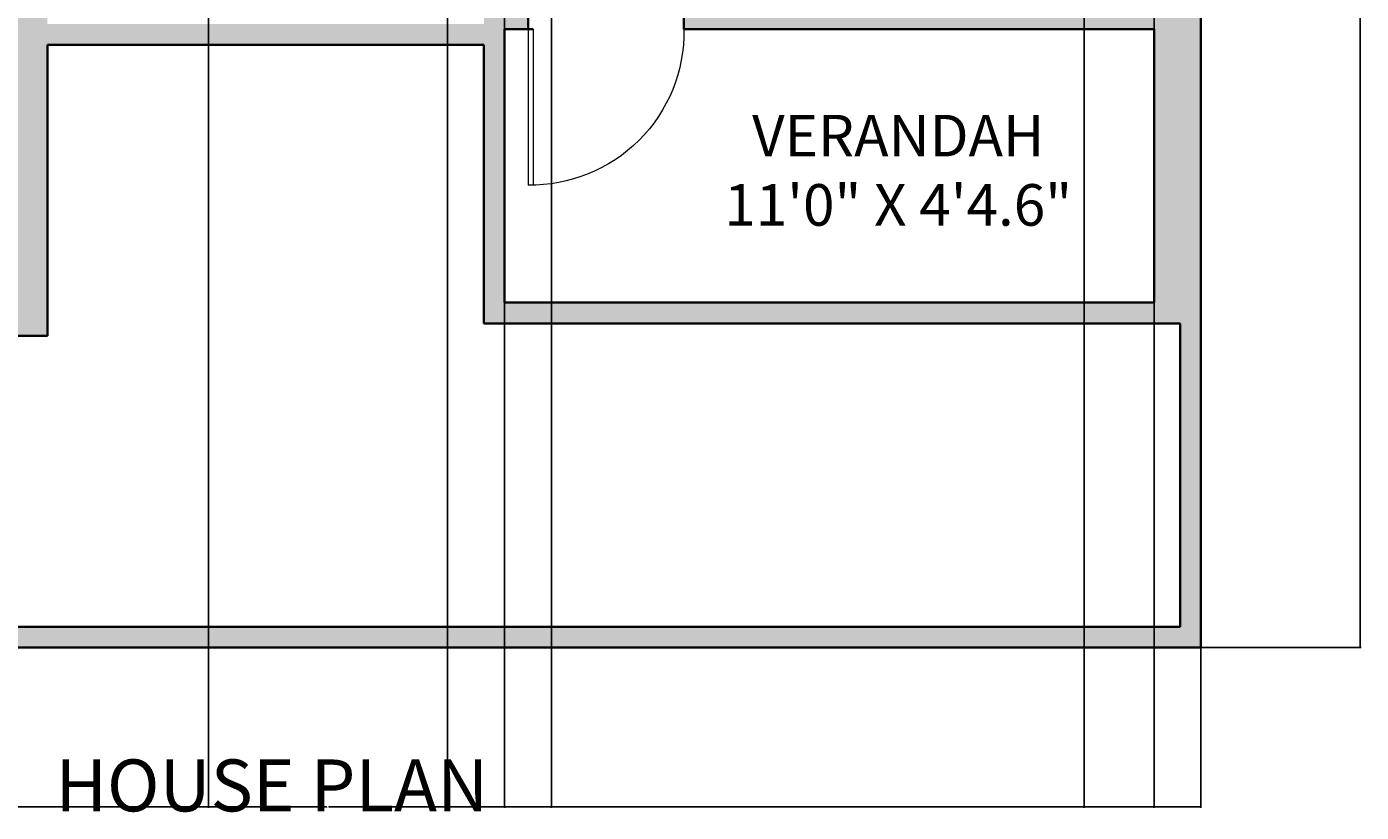
# Model space of a CAD drawing. Units: inches. Extents: x 1567 to 1964, y 1813 to 2447.
# Tile 2 of 28: x 1707 to 1964, y 1813 to 1964. Entities that reach past the tile are written whole.
import ezdxf

# ---------------------------------------------------------------- set-up
doc = ezdxf.new("R2010")
doc.units = ezdxf.units.IN
for name, color, linetype, lineweight in [('A-ANNO-DIMS', 2, 'Continuous', 18), ('A-ANNO-TEXT', 7, 'Continuous', 25), ('A-AREA-IDEN', 7, 'Continuous', 18), ('A-DOOR', 4, 'Continuous', 18), ('A-WALL', 7, 'Continuous', 35)]:
    doc.layers.add(name, color=color, linetype=linetype, lineweight=lineweight)
doc.layers.add('A-WALL-PATT', color=251, linetype='Continuous', lineweight=13, true_color=0x636466)
doc.styles.get("Standard").update_dxf_attribs({"font": 'arial.ttf'})
doc.dimstyles.get("Standard").update_dxf_attribs({"dimtxt": 0.18, "dimasz": 0.18, "dimexe": 0.18, "dimexo": 0.0625, "dimgap": 0.09, "dimtad": 0, "dimtih": 1, "dimtoh": 1, "dimdec": 4, "dimzin": 0, "dimdsep": 46, "dimtxsty": 'Standard', "dimcen": 0.09, "dimadec": 0, "dimazin": 0, "dimtfac": 1, "dimtdec": 4, "dimtofl": 0, "dimtmove": 0, "dimatfit": 3, "dimfxl": 1, "dimtolj": 1, "dimtzin": 0, "dimarcsym": 0})

# ---------------------------------------------------------------- blocks, each defined once
blk = doc.blocks.new('DOOR-SWING-30IN')
for p, q in [((0, 0), (0, 30)), ((1, 0), (1, 30))]:
    blk.add_line(p, q)
blk.add_arc((0.5, 0.5), 29.5, 359.029, 90.971)
blk = doc.blocks.new('*D39')
at = {"layer": 'A-ANNO-DIMS', "color": 0, "lineweight": -2, "transparency": 16777216}
for p, q in [((1597.43, 1844.23), (1597.43, 1813.46)), ((1933.43, 1844.23), (1933.43, 1813.46)), ((1597.61, 1813.64), (1765.14, 1813.64)), ((1933.25, 1813.64), (1765.72, 1813.64))]:
    blk.add_line(p, q, dxfattribs=at)
at = {"layer": 'A-ANNO-DIMS', "color": 0, "transparency": 16777216}
for points in [[(1597.61, 1813.67), (1597.61, 1813.61), (1597.43, 1813.64)], [(1933.25, 1813.67), (1933.25, 1813.61), (1933.43, 1813.64)]]:
    blk.add_solid(points, dxfattribs=at)
at = {"layer": 'Defpoints', "color": 0, "transparency": 16777216}
for p in [(1597.43, 1844.29), (1933.43, 1844.29), (1933.43, 1813.64)]:
    blk.add_point(p, dxfattribs=at)
at = {"layer": 'A-ANNO-DIMS', "color": 0, "transparency": 16777216, "insert": (1765.43, 1813.64), "char_height": 0.18, "attachment_point": 5}
blk.add_mtext('\\A1;336', dxfattribs=at)
blk = doc.blocks.new('*D40')
at = {"layer": 'A-ANNO-DIMS', "color": 0, "lineweight": -2, "transparency": 16777216}
for p, q in [((1933.49, 2416.29), (1964.26, 2416.29)), ((1964.08, 2416.11), (1964.08, 2130.47)), ((1964.08, 1844.47), (1964.08, 2130.11)), ((1933.49, 1844.29), (1964.26, 1844.29))]:
    blk.add_line(p, q, dxfattribs=at)
at = {"layer": 'A-ANNO-DIMS', "color": 0, "transparency": 16777216}
for points in [[(1964.05, 2416.11), (1964.11, 2416.11), (1964.08, 2416.29)], [(1964.05, 1844.47), (1964.11, 1844.47), (1964.08, 1844.29)]]:
    blk.add_solid(points, dxfattribs=at)
at = {"layer": 'Defpoints', "color": 0, "transparency": 16777216}
for p in [(1933.43, 2416.29), (1964.08, 2416.29), (1933.43, 1844.29)]:
    blk.add_point(p, dxfattribs=at)
at = {"layer": 'A-ANNO-DIMS', "color": 0, "transparency": 16777216, "insert": (1964.08, 2130.29), "char_height": 0.18, "attachment_point": 5}
blk.add_mtext('\\A1;572', dxfattribs=at)
blk = doc.blocks.new('*D47')
at = {"layer": 'A-ANNO-DIMS', "color": 0, "lineweight": -2, "transparency": 16777216}
for p, q in [((1742.43, 2331.23), (1742.43, 1813.46)), ((1788.43, 2331.23), (1788.43, 1813.46)), ((1742.61, 1813.64), (1765.21, 1813.64)), ((1788.25, 1813.64), (1765.65, 1813.64))]:
    blk.add_line(p, q, dxfattribs=at)
at = {"layer": 'A-ANNO-DIMS', "color": 0, "transparency": 16777216}
for points in [[(1742.61, 1813.67), (1742.61, 1813.61), (1742.43, 1813.64)], [(1788.25, 1813.67), (1788.25, 1813.61), (1788.43, 1813.64)]]:
    blk.add_solid(points, dxfattribs=at)
at = {"layer": 'Defpoints', "color": 0, "transparency": 16777216}
for p in [(1742.43, 2331.29), (1788.43, 2331.29), (1788.43, 1813.64)]:
    blk.add_point(p, dxfattribs=at)
at = {"layer": 'A-ANNO-DIMS', "color": 0, "transparency": 16777216, "insert": (1765.43, 1813.64), "char_height": 0.18, "attachment_point": 5}
blk.add_mtext('\\A1;46', dxfattribs=at)
blk = doc.blocks.new('*D69')
at = {"layer": 'A-ANNO-DIMS', "color": 0, "lineweight": -2, "transparency": 16777216}
for p, q in [((1799.43, 2123.23), (1799.43, 1813.46)), ((1808.43, 2123.23), (1808.43, 1813.46)), ((1799.61, 1813.64), (1803.78, 1813.64)), ((1808.25, 1813.64), (1804.08, 1813.64))]:
    blk.add_line(p, q, dxfattribs=at)
at = {"layer": 'A-ANNO-DIMS', "color": 0, "transparency": 16777216}
for points in [[(1799.61, 1813.67), (1799.61, 1813.61), (1799.43, 1813.64)], [(1808.25, 1813.67), (1808.25, 1813.61), (1808.43, 1813.64)]]:
    blk.add_solid(points, dxfattribs=at)
at = {"layer": 'Defpoints', "color": 0, "transparency": 16777216}
for p in [(1799.43, 2123.29), (1808.43, 2123.29), (1808.43, 1813.64)]:
    blk.add_point(p, dxfattribs=at)
at = {"layer": 'A-ANNO-DIMS', "color": 0, "transparency": 16777216, "insert": (1803.93, 1813.64), "char_height": 0.18, "attachment_point": 5}
blk.add_mtext('\\A1;9', dxfattribs=at)
blk = doc.blocks.new('*D71')
at = {"layer": 'A-ANNO-DIMS', "color": 0, "lineweight": -2, "transparency": 16777216}
for p, q in [((1799.43, 1910.75), (1799.43, 2447.12)), ((1799.61, 2446.94), (1861.65, 2446.94)), ((1924.25, 2446.94), (1862.21, 2446.94)), ((1924.43, 1910.75), (1924.43, 2447.12))]:
    blk.add_line(p, q, dxfattribs=at)
at = {"layer": 'A-ANNO-DIMS', "color": 0, "transparency": 16777216}
for points in [[(1799.61, 2446.97), (1799.61, 2446.91), (1799.43, 2446.94)], [(1924.25, 2446.97), (1924.25, 2446.91), (1924.43, 2446.94)]]:
    blk.add_solid(points, dxfattribs=at)
at = {"layer": 'Defpoints', "color": 0, "transparency": 16777216}
for p in [(1924.43, 2446.94), (1799.43, 1910.69), (1924.43, 1910.69)]:
    blk.add_point(p, dxfattribs=at)
at = {"layer": 'A-ANNO-DIMS', "color": 0, "transparency": 16777216, "insert": (1861.93, 2446.94), "char_height": 0.18, "attachment_point": 5}
blk.add_mtext('\\A1;125', dxfattribs=at)
blk = doc.blocks.new('*D72')
at = {"layer": 'A-ANNO-DIMS', "color": 0, "lineweight": -2, "transparency": 16777216}
for p, q in [((1910.93, 2175.23), (1910.93, 1813.46)), ((1924.43, 2175.23), (1924.43, 1813.46)), ((1911.11, 1813.64), (1917.36, 1813.64)), ((1924.25, 1813.64), (1918, 1813.64))]:
    blk.add_line(p, q, dxfattribs=at)
at = {"layer": 'A-ANNO-DIMS', "color": 0, "transparency": 16777216}
for points in [[(1911.11, 1813.67), (1911.11, 1813.61), (1910.93, 1813.64)], [(1924.25, 1813.67), (1924.25, 1813.61), (1924.43, 1813.64)]]:
    blk.add_solid(points, dxfattribs=at)
at = {"layer": 'Defpoints', "color": 0, "transparency": 16777216}
for p in [(1910.93, 2175.29), (1924.43, 2175.29), (1924.43, 1813.64)]:
    blk.add_point(p, dxfattribs=at)
at = {"layer": 'A-ANNO-DIMS', "color": 0, "transparency": 16777216, "insert": (1917.68, 1813.64), "char_height": 0.18, "attachment_point": 5}
blk.add_mtext('\\A1;13.5', dxfattribs=at)

msp = doc.modelspace()

# ---------------------------------------------------------------- hatches: boundary and pattern name
at = {"layer": 'A-WALL-PATT'}
h = msp.add_hatch(color=256, dxfattribs=at)
h.dxf.hatch_style = 1
h.paths.add_polyline_path([(1606.4295, 2407.29), (1654.4295, 2407.29), (1654.4295, 2416.29), (1597.4295, 2416.29), (1597.4295, 2217.29), (1606.4295, 2217.29), (1606.4295, 2259.29), (1738.4295, 2259.29), (1738.4295, 2247.29), (1742.4295, 2247.29), (1742.4295, 2259.29), (1742.4295, 2272.29), (1738.4295, 2272.29), (1738.4295, 2263.29), (1606.4295, 2263.29)])
h.paths.add_polyline_path([(1753.4295, 2416.29), (1690.4295, 2416.29), (1690.4295, 2407.29), (1738.4295, 2407.29), (1738.4295, 2308.29), (1742.4295, 2308.29), (1742.4295, 2331.29), (1746.9295, 2331.29), (1746.9295, 2335.29), (1742.4295, 2335.29), (1742.4295, 2407.29), (1753.4295, 2407.29)])
h.paths.add_polyline_path([(1840.4295, 2416.29), (1777.4295, 2416.29), (1777.4295, 2407.29), (1788.4295, 2407.29), (1788.4295, 2335.29), (1776.9295, 2335.29), (1776.9295, 2331.29), (1788.4295, 2331.29), (1788.4295, 2308.29), (1792.4295, 2308.29), (1792.4295, 2407.29), (1840.4295, 2407.29)])
h.paths.add_polyline_path([(1933.4295, 2416.29), (1876.4295, 2416.29), (1876.4295, 2407.29), (1924.4295, 2407.29), (1924.4295, 2263.29), (1792.4295, 2263.29), (1792.4295, 2272.29), (1788.4295, 2272.29), (1788.4295, 2259.29), (1872.4295, 2259.29), (1872.4295, 2171.29), (1880.9295, 2171.29), (1880.9295, 2175.29), (1876.4295, 2175.29), (1876.4295, 2259.29), (1924.4295, 2259.29), (1924.4295, 2229.29), (1933.4295, 2229.29)])
h.paths.add_polyline_path([(1933.4295, 2205.29), (1924.4295, 2205.29), (1924.4295, 2175.29), (1910.9295, 2175.29), (1910.9295, 2171.29), (1924.4295, 2171.29), (1924.4295, 2127.29), (1844.4295, 2127.29), (1844.4295, 2123.29), (1924.4295, 2123.29), (1924.4295, 2063.29), (1933.4295, 2063.29)])
h.paths.add_polyline_path([(1799.4295, 2123.29), (1808.4295, 2123.29), (1808.4295, 2127.29), (1781.4295, 2127.29), (1781.4295, 2123.29), (1795.4295, 2123.29), (1795.4295, 1964.29), (1711.4295, 1964.29), (1711.4295, 2123.29), (1751.4295, 2123.29), (1751.4295, 2127.29), (1742.4295, 2127.29), (1742.4295, 2139.29), (1738.4295, 2139.29), (1738.4295, 2127.29), (1678.4295, 2127.29), (1678.4295, 2123.29), (1702.4295, 2123.29), (1702.4295, 1913.29), (1678.4295, 1913.29), (1678.4295, 1904.29), (1711.4295, 1904.29), (1711.4295, 1960.29), (1795.4295, 1960.29), (1795.4295, 1906.69), (1929.4295, 1906.69), (1929.4295, 1848.29), (1601.4295, 1848.29), (1601.4295, 1904.29), (1630.4295, 1904.29), (1630.4295, 1913.29), (1606.4295, 1913.29), (1606.4295, 2123.29), (1630.4295, 2123.29), (1630.4295, 2127.29), (1606.4295, 2127.29), (1606.4295, 2169.29), (1597.4295, 2169.29), (1597.4295, 1844.29), (1933.4295, 1844.29), (1933.4295, 2027.29), (1924.4295, 2027.29), (1924.4295, 1967.29), (1833.9295, 1967.29), (1833.9295, 1963.29), (1924.4295, 1963.29), (1924.4295, 1910.69), (1799.4295, 1910.69), (1799.4295, 1963.29), (1803.9295, 1963.29), (1803.9295, 1967.29), (1799.4295, 1967.29)])

# ---------------------------------------------------------------- linework, layer by layer
at = {"layer": 'A-WALL'}
for p, q in [((1933.4295, 2416.29), (1933.4295, 1844.29)), ((1803.9295, 1967.29), (1803.9295, 1963.29)), ((1833.9295, 1963.29), (1833.9295, 1967.29)), ((1799.4295, 1910.69), (1799.4295, 1963.29)), ((1804.9295, 1963.29), (1799.4295, 1963.29)), ((1924.4295, 1963.29), (1833.9295, 1963.29)), ((1924.4295, 1963.29), (1924.4295, 1910.69)), ((1711.4295, 1904.29), (1711.4295, 1960.29)), ((1711.4295, 1960.29), (1795.4295, 1960.29)), ((1795.4295, 1906.69), (1795.4295, 1960.29)), ((1924.4295, 1910.69), (1799.4295, 1910.69)), ((1929.4295, 1906.69), (1795.4295, 1906.69)), ((1929.4295, 1906.69), (1929.4295, 1848.29)), ((1601.4295, 1904.29), (1711.4295, 1904.29)), ((1601.4295, 1848.29), (1929.4295, 1848.29)), ((1597.4295, 1844.29), (1933.4295, 1844.29))]:
    msp.add_line(p, q, dxfattribs=at)

# ---------------------------------------------------------------- block references
at = {"layer": 'A-DOOR', "extrusion": (0, 0, -1), "zscale": -1, "rotation": 180}
msp.add_blockref('DOOR-SWING-30IN', (-1803.93, 1963.29), dxfattribs=at)

# ---------------------------------------------------------------- texts
at = {"layer": 'A-ANNO-TEXT', "insert": (1712.9667, 1822.7547), "char_height": 10, "attachment_point": 1}
msp.add_mtext_dynamic_manual_height_columns('{\\fArial|b1|i0|c0|p34;HOUSE PLAN}', width=163.150734, gutter_width=12.5, heights=[0], dxfattribs=at)
at = {"layer": 'A-AREA-IDEN', "insert": (1834.2874, 1946.8199), "char_height": 8, "attachment_point": 1}
msp.add_mtext_dynamic_manual_height_columns('\\pxqc;VERANDAH\\P11\'0" X 4\'4.6"', width=81.753814, gutter_width=12.5, heights=[0], dxfattribs=at)

# ---------------------------------------------------------------- dimensions: what is measured, and where the dimension line sits
at = {"layer": 'A-ANNO-DIMS'}
for base, p1, p2, override, picture, middle in [((1924.4295, 2446.94), (1799.4295, 1910.69), (1924.4295, 1910.69), {"dimdec": 0, "dimlfac": 1, "dimrnd": 0, "dimzin": 0, "dimdsep": 46, "dimlunit": 2}, '*D71', (1861.9295, 2446.94)), ((1788.4295, 1813.64), (1742.4295, 2331.29), (1788.4295, 2331.29), {"dimdec": 0, "dimlfac": 1, "dimrnd": 0, "dimzin": 0, "dimdsep": 46, "dimlunit": 2}, '*D47', (1765.4295, 1813.64)), ((1924.4295, 1813.64), (1910.9295, 2175.29), (1924.4295, 2175.29), {"dimdec": 1, "dimlfac": 1, "dimrnd": 0, "dimzin": 0, "dimdsep": 46, "dimlunit": 2}, '*D72', (1917.6795, 1813.64)), ((1808.4295, 1813.64), (1799.4295, 2123.29), (1808.4295, 2123.29), {"dimdec": 0, "dimlfac": 1, "dimrnd": 0, "dimzin": 0, "dimdsep": 46, "dimlunit": 2}, '*D69', (1803.9295, 1813.64)), ((1933.4295, 1813.64), (1597.4295, 1844.29), (1933.4295, 1844.29), {"dimdec": 0, "dimlfac": 1, "dimrnd": 0, "dimzin": 0, "dimdsep": 46, "dimlunit": 2}, '*D39', (1765.4295, 1813.64))]:
    dim = msp.add_linear_dim(base=base, p1=p1, p2=p2, dimstyle='Standard', override=override, dxfattribs=at)
    dim.commit()
    dim.dimension.update_dxf_attribs({"geometry": picture, "text_midpoint": middle})
dim = msp.add_linear_dim(base=(1964.0795, 2416.29), p1=(1933.4295, 1844.29), p2=(1933.4295, 2416.29), angle=90, dimstyle='Standard', override={"dimdec": 0, "dimlfac": 1, "dimrnd": 0, "dimzin": 0, "dimdsep": 46, "dimlunit": 2}, dxfattribs=at)
dim.commit()
dim.dimension.update_dxf_attribs({"geometry": '*D40', "text_midpoint": (1964.0795, 2130.29)})

doc.saveas('drawing.dxf')
